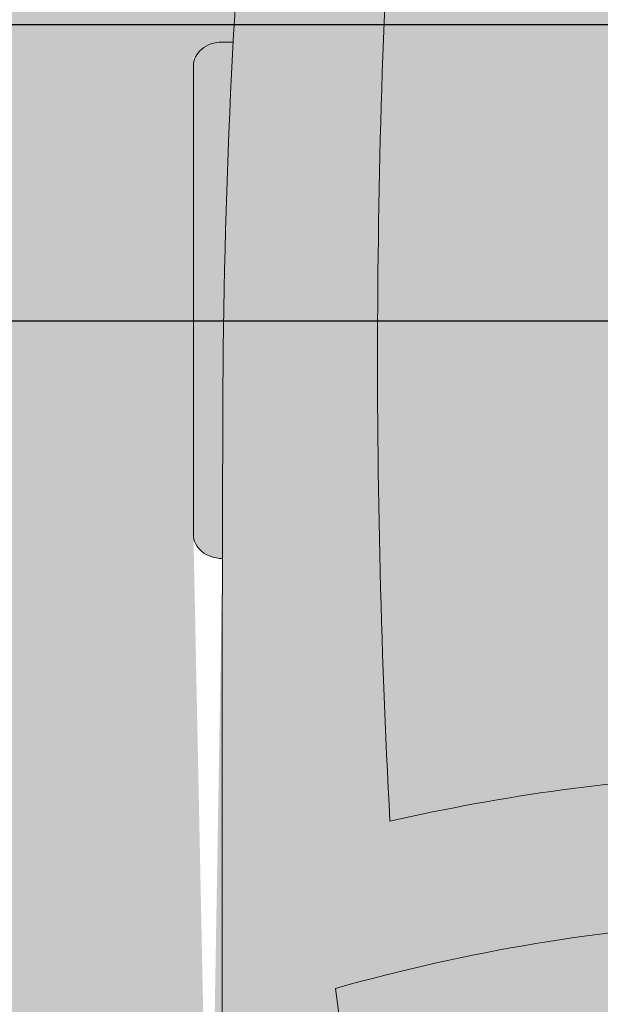
# Model space of a CAD drawing. Units: inches. Extents: x 389 to 971, y 148 to 870.
# Tile 2 of 14: x 477 to 500, y 349 to 389. Entities that reach past the tile are written whole.
import ezdxf

# ---------------------------------------------------------------- set-up
doc = ezdxf.new("R2010")
doc.units = ezdxf.units.IN
doc.header["$MEASUREMENT"] = 0
for name, color, linetype, lineweight in [('A-ANNO-DIMS', 2, 'Continuous', 18), ('C-VEHI', 8, 'Continuous', 13), ('L-GRND-BASE-PATT', 8, 'Continuous', 13)]:
    doc.layers.add(name, color=color, linetype=linetype, lineweight=lineweight)
doc.layers.add('C-VEHI-PATT', color=18, linetype='Continuous', lineweight=13, true_color=0x000000)
doc.layers.add('L-GRND-PATT', color=39, linetype='Continuous', lineweight=13, true_color=0x603913)
doc.styles.get("Standard").update_dxf_attribs({"font": 'arial.ttf'})
doc.dimstyles.get("Standard").update_dxf_attribs({"dimtxt": 8, "dimasz": 8, "dimexe": 0.18, "dimexo": 0.0625, "dimgap": 0.09, "dimtad": 0, "dimtih": 1, "dimtoh": 1, "dimdec": 0, "dimzin": 0, "dimdsep": 46, "dimlunit": 3, "dimtxsty": 'Standard', "dimcen": 0.09, "dimadec": 0, "dimazin": 0, "dimtfac": 1, "dimtdec": 0, "dimtofl": 0, "dimtmove": 0, "dimatfit": 3, "dimfxl": 1, "dimtolj": 1, "dimtzin": 0, "dimarcsym": 0})

# ---------------------------------------------------------------- blocks, each defined once
blk = doc.blocks.new('*U7')
for p, q in [((86.40615155322318, -29.35124891408145), (70.03028248535594, -31.53613089391442)), ((21.10406751471477, -37.4086304679212), (21.10406751471477, -36.83230215753756)), ((47.80016686962392, -37.39011648242107), (47.80016686962392, -37.4086304679212)), ((46.55368679439944, -38.88847654282927), (22.35054758993934, -38.88847654282927))]:
    blk.add_line(p, q)
for centre, major_axis, ratio, start_param, end_param in [((135.2911776514465, -5.387441675480715), (3.2038e-12, -81.77258453066244), 0.8423038695439492, -1.50788012981387, -1.245306111696839), ((134.4003789125684, -5.387441675478584), (4.2949e-12, -89.77745434847827), 0.8423038695439354, -1.510751403667474, -1.307889310215002), ((37.47375371777847, 593.9621830607904), (1.1693e-12, -623.3282099673584), 0.8423038695439528, -0.0593185269054384, 0.0455465850287298), ((41.19115208863322, 490.8631038926152), (1.37757e-11, -528.2339998381949), 0.8423038695440652, -0.0755983031097181, -0.0028100083537155), ((64.48199294495228, 10555.61767590795), (6.117947e-10, 10593.02630637587), 0.8423038695458146, 3.138795612625926, 3.154989602201039), ((22.35054758993934, -37.40863046792117), (2.2e-14, 1.479846074908118), 0.8423038695439758, 1.570796326794908, 3.14159265358981), ((46.55368679439944, -37.40863046792117), (2.08e-14, -1.479846074908118), 0.842303869543976, -1.69e-14, 1.570796326794884)]:
    blk.add_ellipse(centre, major_axis=major_axis, ratio=ratio, start_param=start_param, end_param=end_param)
blk = doc.blocks.new('*D53')
at = {"layer": 'A-ANNO-DIMS', "color": 0, "lineweight": -2, "transparency": 16777216}
for p, q in [((397.8910240000004, 396.9189020000002), (397.8910240000004, 404.9189020000001)), ((690.1535240000002, 388.9189020000003), (397.7110240000004, 388.9189020000002)), ((690.1535240000002, 376.9189020000001), (397.7110240000005, 376.9189020000001)), ((397.8910240000005, 368.9189020000001), (397.8910240000005, 360.918902))]:
    blk.add_line(p, q, dxfattribs=at)
at = {"layer": 'A-ANNO-DIMS', "color": 0, "transparency": 16777216}
for points in [[(396.5576906666671, 396.9189020000002), (399.2243573333337, 396.9189020000002), (397.8910240000004, 388.9189020000002)], [(396.5576906666671, 368.9189020000001), (399.2243573333338, 368.9189020000001), (397.8910240000005, 376.9189020000001)]]:
    blk.add_solid(points, dxfattribs=at)
at = {"layer": 'Defpoints', "color": 0, "transparency": 16777216}
for p in [(397.8910240000004, 388.9189020000002), (690.2160240000001, 388.9189020000003), (690.2160240000001, 376.9189020000001)]:
    blk.add_point(p, dxfattribs=at)
at = {"layer": 'A-ANNO-DIMS', "color": 0, "transparency": 16777216, "insert": (397.8910240000004, 382.9189019999999), "char_height": 8, "attachment_point": 5}
blk.add_mtext('\\A1;12', dxfattribs=at)

msp = doc.modelspace()

# ---------------------------------------------------------------- hatches: boundary and pattern name
at = {"layer": 'C-VEHI-PATT'}
h = msp.add_hatch(color=256, dxfattribs=at)
h.dxf.hatch_style = 1
edge = h.paths.add_edge_path()
edge.add_ellipse((550.9021553826709, 381.4331108862803), major_axis=(-43.99405423656321, 1.9369e-12), ratio=0.8423038695439613, start_angle=-29.43856959797762, end_angle=1.8189894035458565e-12, ccw=False)
edge.add_line((514.3535105156315, 402.059641051582), (514.3535105156315, 404.7525403567118))
edge.add_ellipse((514.3535105156316, 404.2643898676136), major_axis=(0.5795420236673633, 2e-16), ratio=0.8423038695437671, start_angle=90.00000000001334, end_angle=127.9331304598466)
edge.add_line((514.0354569934393, 404.6724605914631), (509.5535496243029, 402.1940957519602))
edge.add_ellipse((473.3138688667988, 564.9222417143382), major_axis=(196.5636751472093, 8.4793e-12), ratio=0.8423038695439335, start_angle=-80.7434339928015, end_angle=-77.44506735586577, ccw=False)
edge.add_ellipse((535.9119176052684, 201.7546502845751), major_axis=(239.1273775699096, 1.008988e-10), ratio=0.842303869543627, start_angle=100.2095389971183, end_angle=102.4446272934191)
edge.add_ellipse((979.5722266908713, 375.4013592680145), major_axis=(-488.2195497741742, 7.7268e-12), ratio=0.842303869543895, start_angle=-2.863714607837472, end_angle=2.198540565955285)
edge.add_ellipse((510.1338164488812, 299.4839331720496), major_axis=(70.3178640738586, 3.814e-12), ratio=0.8423038695439212, start_angle=94.08241069114638, end_angle=107.71995322274631, ccw=False)
edge.add_line((505.914122382133, 358.6062023341113), (522.79289864913, 358.606202334111))
edge.add_ellipse((518.5732045823792, 299.4839331720493), major_axis=(-70.31786407385354, 1.4408e-12), ratio=0.8423038695439844, start_angle=252.2800467772501, end_angle=265.91758930884987, ccw=False)
edge.add_ellipse((49.13479434038987, 375.4013592680261), major_axis=(-488.2195497741754, 2.5232e-12), ratio=0.8423038695439587, start_angle=177.8014594340444, end_angle=182.8637146078372)
edge.add_ellipse((492.795103425985, 201.7546502845724), major_axis=(239.12737756976, 4.82267e-11), ratio=0.8423038695441539, start_angle=77.5553727065425, end_angle=79.79046100284327)
edge.add_ellipse((555.3931521644682, 564.9222417143374), major_axis=(-196.5636751472384, 3.62381e-11), ratio=0.8423038695438114, start_angle=77.4450673558726, end_angle=80.74343399280832, ccw=False)
edge.add_line((519.1534714069603, 402.19409575196), (514.671564037824, 404.6724605914631))
edge.add_ellipse((514.3535105156316, 404.2643898676136), major_axis=(0.5795420236673633, 2e-16), ratio=0.8423038695437671, start_angle=52.06686954015338, end_angle=90.00000000001334)
edge.add_line((514.3535105156315, 404.7525403567118), (514.3535105156315, 402.0596410515821))
edge.add_ellipse((477.8048656485917, 381.4331108862812), major_axis=(-43.99405423656326, 6.67e-13), ratio=0.8423038695439753, start_angle=180.0000000000002, end_angle=209.4385695979796, ccw=False)
edge.add_line((521.7989198851549, 381.4331108862806), (521.7989198851549, 379.5923831537828))
edge.add_line((521.7989198851549, 379.5923831537828), (523.2258361412675, 379.5923831537828))
edge.add_ellipse((523.0896049791924, 379.1042326646847), major_axis=(0.5795420236669786, 3.601e-13), ratio=0.8423038695443263, start_angle=45.519789117397124, end_angle=89.99999999996442, ccw=False)
edge.add_line((523.4589887688404, 379.4803801228631), (527.8015488731598, 376.4548385069232))
edge.add_line((527.8015488731598, 376.4548385069232), (527.8015488731597, 364.8548231745798))
edge.add_ellipse((524.8002343791572, 364.9712406163019), major_axis=(0.279312372030448, 4.96584264291768), ratio=0.6038335755719146, start_angle=106.34259195429831, end_angle=270.9979857249735, ccw=False)
edge.add_line((521.7989198851548, 364.2715269884119), (521.7989198851549, 381.4331108862806))
edge.add_ellipse((477.8048656485917, 381.4331108862812), major_axis=(-43.99405423656326, 6.67e-13), ratio=0.8423038695439753, start_angle=180.0000000000001, end_angle=209.4385695979795)
edge.add_ellipse((550.9021553826709, 381.4331108862803), major_axis=(-43.99405423656321, 1.9369e-12), ratio=0.8423038695439613, start_angle=-29.43856959797755, end_angle=1.8539e-12)
edge.add_line((506.9081011461076, 381.43311088628), (506.9081011461074, 364.2715269884121))
edge.add_ellipse((503.9067866521049, 364.9712406163021), major_axis=(-0.2793123720310282, 4.965842642917721), ratio=0.6038335755718928, start_angle=89.00201427501901, end_angle=253.6574080456941, ccw=False)
edge.add_line((500.9054721581025, 364.8548231745812), (500.9054721581025, 376.4548385069235))
edge.add_line((500.9054721581025, 376.4548385069235), (505.3530060491612, 379.5535172937331))
edge.add_ellipse((505.61741605207, 379.1042326646849), major_axis=(-0.5795420236672051, 1.236e-13), ratio=0.842303869543997, start_angle=-89.99999999998778, end_angle=-45.51978911742469, ccw=False)
edge.add_line((505.61741605207, 379.5923831537831), (506.9081011461076, 379.5923831537831))
edge.add_line((506.9081011461076, 379.5923831537831), (506.9081011461076, 381.43311088628))
h = msp.add_hatch(color=256, dxfattribs=at)
h.dxf.hatch_style = 1
edge = h.paths.add_edge_path()
edge.add_ellipse((550.9021553826709, 381.4331108862803), major_axis=(-43.99405423656321, 1.9369e-12), ratio=0.8423038695439613, start_angle=-17.01851281727818, end_angle=1.8189894035458565e-12, ccw=False)
edge.add_line((509.5535496243029, 394.0892586662828), (509.5535496243029, 402.1940957519602))
edge.add_ellipse((473.3138688667988, 564.9222417143382), major_axis=(196.5636751472093, 8.4793e-12), ratio=0.8423038695439335, start_angle=-80.7434339928015, end_angle=-77.44506735586577, ccw=False)
edge.add_ellipse((535.9119176052684, 201.7546502845751), major_axis=(239.1273775699096, 1.008988e-10), ratio=0.842303869543627, start_angle=100.2095389971183, end_angle=102.4446272934191)
edge.add_ellipse((979.5722266908713, 375.4013592680145), major_axis=(-488.2195497741742, 7.7268e-12), ratio=0.842303869543895, start_angle=-2.863714607837472, end_angle=2.198540565955285)
edge.add_ellipse((510.1338164488812, 299.4839331720496), major_axis=(70.3178640738586, 3.814e-12), ratio=0.8423038695439212, start_angle=94.08241069114638, end_angle=107.71995322274631, ccw=False)
edge.add_line((505.914122382133, 358.6062023341113), (509.5535496243029, 358.6062023341112))
edge.add_line((509.5535496243029, 358.6062023341112), (509.5535496243029, 394.0892586662828))
edge.add_ellipse((550.9021553826709, 381.4331108862803), major_axis=(-43.99405423656321, 1.9369e-12), ratio=0.8423038695439613, start_angle=-17.01851281727824, end_angle=1.8539e-12)
edge.add_line((506.9081011461076, 381.43311088628), (506.9081011461074, 364.2715269884121))
edge.add_ellipse((503.9067866521049, 364.9712406163021), major_axis=(-0.2793123720310282, 4.965842642917721), ratio=0.6038335755718928, start_angle=89.00201427501901, end_angle=253.6574080456941, ccw=False)
edge.add_line((500.9054721581025, 364.8548231745812), (500.9054721581025, 376.4548385069235))
edge.add_line((500.9054721581025, 376.4548385069235), (505.3172273641584, 379.5285896248376))
edge.add_ellipse((505.61741605207, 379.1042326646849), major_axis=(-0.5795420236672051, 1.236e-13), ratio=0.842303869543997, start_angle=-89.99999999998778, end_angle=-45.51978911742469, ccw=False)
edge.add_line((505.61741605207, 379.5923831537831), (506.9081011461076, 379.5923831537831))
edge.add_line((506.9081011461076, 379.5923831537831), (506.9081011461076, 381.43311088628))
h = msp.add_hatch(color=256, dxfattribs=at)
h.dxf.hatch_style = 1
edge = h.paths.add_edge_path(flags=16)
edge.add_ellipse((3386.011413077446, 329.726312794031), major_axis=(-2896.629999631248, 1.069454e-10), ratio=0.8423038695494893, start_angle=-0.1208973690315247, end_angle=0.3640763488915013, ccw=False)
edge.add_line((489.3905023836935, 335.8383575186984), (486.2179253655185, 346.1978202249628))
edge.add_ellipse((8782.002602781096, 354.247254279773), major_axis=(-8295.790181758603, 9.87839e-10), ratio=0.8423038695486498, start_angle=0.0555943135052214, end_angle=0.3777641939157137)
edge.add_line((486.4665645878948, 299.5520931219791), (489.4638383140943, 311.3204429697198))
edge = h.paths.add_edge_path(flags=16)
edge.add_ellipse((512.1608573463288, 287.5825181681774), major_axis=(62.33048198263887, 2.0798e-12), ratio=0.8423038695439498, start_angle=94.8700695971331, end_angle=112.791914877584)
edge.add_line((491.3642517254777, 337.0752369161335), (489.6529508739416, 349.9015767089268))
edge.add_ellipse((510.1338164488795, 298.7862183048575), major_axis=(64.04807894948699, 3.9006e-12), ratio=0.8423038695439252, start_angle=94.27742096304979, end_angle=111.83495379670401, ccw=False)
edge.add_line((506.1068129054811, 352.6274231954524), (522.600208125781, 352.6274231954521))
edge.add_ellipse((518.5732045823798, 298.7862183048586), major_axis=(64.04807894948067, 3.24e-14), ratio=0.8423038695439885, start_angle=68.16504620328948, end_angle=85.72257903694378, ccw=False)
edge.add_line((539.05407015732, 349.9015767089259), (537.3427693057835, 337.0752369161327))
edge.add_ellipse((516.5461636849332, 287.5825181681899), major_axis=(62.33048198262021, 1.5954e-12), ratio=0.8423038695439995, start_angle=67.20808512240782, end_angle=85.12993040286212)
edge.add_line((521.0080028322477, 339.9490379899644), (507.6990181990146, 339.9490379899646))
edge = h.paths.add_edge_path(flags=16)
edge.add_ellipse((514.3535105156315, 391.3730654902235), major_axis=(-115.1512533244504, 1.8736e-12), ratio=0.8423038695439684, start_angle=76.4018653097696, end_angle=103.5981346902308)
edge.add_line((537.3427693057832, 296.3333211885938), (537.342769305783, 281.5897392316151))
edge.add_ellipse((514.3535105156313, 376.6294835332447), major_axis=(-115.1512533244486, 9.02e-13), ratio=0.8423038695439828, start_angle=76.40186530976922, end_angle=103.59813469023032, ccw=False)
edge.add_line((491.3642517254773, 281.5897392316156), (491.3642517254774, 296.3333211885945))
edge = h.paths.add_edge_path()
edge.add_ellipse((8782.002602781105, 354.2472542798386), major_axis=(-8296.949265805946, 5.39345e-11), ratio=0.8423038695428886, start_angle=0.3838667787920247, end_angle=0.5282714718170651)
edge.add_ellipse((8782.002602781105, 354.2472542798386), major_axis=(-8296.949265805946, 5.39345e-11), ratio=0.8423038695428886, start_angle=0.5282714718170651, end_angle=0.6465540970606384)
edge.add_ellipse((488.1158467995968, 260.6509346628684), major_axis=(2.318168094668909, 7.48e-14), ratio=0.8423038695439647, start_angle=180.6465540970884, end_angle=269.9999999999081)
edge.add_line((488.115846799593, 258.6983327064755), (491.3642517254771, 258.6983327064753))
edge.add_line((491.3642517254771, 258.6983327064753), (491.3642517254771, 274.201106836649))
edge.add_ellipse((493.6824198201462, 273.9438556676354), major_axis=(-2.318168094668919, 1.896e-13), ratio=0.8423038695439611, start_angle=-89.99999999999523, end_angle=4.718003765447065e-12, ccw=False)
edge.add_line((493.6824198201462, 275.8964576240284), (535.3300149439905, 275.8964576240277))
edge.add_ellipse((535.024601211114, 273.9438556676347), major_axis=(2.318168094668976, 2.946e-13), ratio=0.8423038695439647, start_angle=-7.275957614183426e-12, end_angle=89.99999999998943, ccw=False)
edge.add_line((537.342769305783, 273.9438556676347), (537.3427693057827, 258.698332706474))
edge.add_line((537.3427693057827, 258.698332706474), (540.591174231666, 258.6983327064739))
edge.add_ellipse((540.5911742316634, 260.6509346628669), major_axis=(-2.318168094668839, 2.143e-13), ratio=0.8423038695440144, start_angle=90.00000000008203, end_angle=179.3534459029346)
edge.add_ellipse((-7753.295581726658, 354.2472542799028), major_axis=(-8296.949265782761, 2.068448e-10), ratio=0.8423038695442414, start_angle=179.3534459029388, end_angle=179.3813568036815)
edge.add_ellipse((-7753.295581726658, 354.2472542799028), major_axis=(-8296.949265782761, 2.068448e-10), ratio=0.8423038695442414, start_angle=179.3813568036815, end_angle=179.4717285281828)
edge.add_ellipse((-7753.295581726658, 354.2472542799028), major_axis=(-8296.949265782761, 2.068448e-10), ratio=0.8423038695442414, start_angle=179.4717285281828, end_angle=179.6161332212082)
edge.add_ellipse((-7753.295581726658, 354.2472542799028), major_axis=(-8296.949265782761, 2.068448e-10), ratio=0.8423038695442414, start_angle=179.6161332212082, end_angle=180.090229088595)
edge.add_ellipse((-7753.295581726658, 354.2472542799028), major_axis=(-8296.949265782761, 2.068448e-10), ratio=0.8423038695442414, start_angle=180.090229088595, end_angle=180.134986576859)
edge.add_ellipse((129.8867725257751, 372.4897205359271), major_axis=(-413.7373561031673, 2.44623e-11), ratio=0.8423038695441432, start_angle=180.1806905311865, end_angle=182.1799503136479)
edge.add_ellipse((129.8867725257751, 372.4897205359271), major_axis=(-413.7373561031673, 2.44623e-11), ratio=0.8423038695441432, start_angle=182.1799503136479, end_angle=183.6504275857017)
edge.add_ellipse((492.7951034259847, 196.3854951855023), major_axis=(245.3971626940514, 1.422861e-10), ratio=0.8423038695444116, start_angle=76.21947101046817, end_angle=77.87403444768196)
edge.add_ellipse((49.13479434038987, 375.4013592680261), major_axis=(-488.2195497741754, 2.5232e-12), ratio=0.8423038695439587, start_angle=177.8014594340445, end_angle=182.8637146078372, ccw=False)
edge.add_ellipse((518.5732045823792, 299.4839331720493), major_axis=(-70.31786407385354, 1.4408e-12), ratio=0.8423038695439844, start_angle=252.2800467772501, end_angle=265.9175893088498)
edge.add_line((522.79289864913, 358.606202334111), (505.9141223821329, 358.6062023341113))
edge.add_ellipse((510.1338164488812, 299.4839331720496), major_axis=(70.3178640738586, 3.814e-12), ratio=0.8423038695439212, start_angle=94.08241069114636, end_angle=107.7199532227462)
edge.add_ellipse((979.5722266908713, 375.4013592680145), major_axis=(-488.2195497741742, 7.7268e-12), ratio=0.842303869543895, start_angle=-2.863714607837494, end_angle=2.198540565955284, ccw=False)
edge.add_ellipse((535.9119176052733, 196.3854951855018), major_axis=(-245.3971626940985, 1.013648e-10), ratio=0.8423038695442548, start_angle=-77.87403444769295, end_angle=-76.2194710104792)
edge.add_ellipse((898.8202485054873, 372.489720535918), major_axis=(413.7373561031672, 1.26113e-11), ratio=0.8423038695441164, start_angle=176.3495724142985, end_angle=177.8200496863523)
edge.add_ellipse((898.8202485054873, 372.489720535918), major_axis=(413.7373561031672, 1.26113e-11), ratio=0.8423038695441164, start_angle=177.8200496863523, end_angle=179.8643876095591)
edge.add_ellipse((8782.002602781105, 354.2472542798386), major_axis=(-8296.949265805946, 5.39345e-11), ratio=0.8423038695428886, start_angle=-0.1349865768573029, end_angle=-0.090229088593484)
edge.add_ellipse((8782.002602781105, 354.2472542798386), major_axis=(-8296.949265805946, 5.39345e-11), ratio=0.8423038695428886, start_angle=-0.090229088593484, end_angle=0.3838667787920247)
edge = h.paths.add_edge_path(flags=16)
edge.add_ellipse((-2357.304392046186, 329.7263127941099), major_axis=(2896.629999631251, 5.35614e-11), ratio=0.8423038695445265, start_angle=-0.3640763488920631, end_angle=0.1208973690309369)
edge.add_line((539.3165186475693, 335.8383575187012), (542.4890956657468, 346.1978202249727))
edge.add_ellipse((-7753.295581749842, 354.2472542800017), major_axis=(8295.790181758617, 3.2664368e-09), ratio=0.8423038695525207, start_angle=-0.37776419393310334, end_angle=-0.055594313522590255, ccw=False)
edge.add_line((542.240456443367, 299.5520931219743), (539.2431827171666, 311.3204429697195))
h = msp.add_hatch(color=256, dxfattribs=at)
h.dxf.hatch_style = 1
edge = h.paths.add_edge_path()
edge.add_ellipse((898.8202485054873, 372.489720535918), major_axis=(413.7373561031672, 1.26113e-11), ratio=0.8423038695441164, start_angle=177.8200496863524, end_angle=179.8643876095592, ccw=False)
edge.add_line((485.5047440247956, 388.2228563544795), (485.0533369751571, 388.2228563544795))
edge.add_ellipse((485.0533369751571, 387.2465553762829), major_axis=(1.159084047334488, 1.838e-13), ratio=0.8423038695439892, start_angle=89.9999999999909, end_angle=179.9999999999909)
edge.add_line((483.8942529278225, 387.2465553762829), (483.8942529278224, 368.2895347624687))
edge.add_ellipse((485.0533369751568, 368.2895347624687), major_axis=(-1.159084047334488, 1.838e-13), ratio=0.8423038695439892, start_angle=9.0871e-12, end_angle=90.00000000000905)
edge.add_line((485.0533369751553, 367.3132337842722), (485.0678379868568, 367.3132337842722))
edge.add_ellipse((8782.002602781105, 354.2472542798386), major_axis=(-8296.949265805946, 5.39345e-11), ratio=0.8423038695428886, start_angle=-0.13498657685727267, end_angle=-0.0902290885933894, ccw=False)
h = msp.add_hatch(color=256, dxfattribs=at)
h.dxf.hatch_style = 1
edge = h.paths.add_edge_path()
edge.add_ellipse((518.5732045823798, 298.7862183048586), major_axis=(64.04807894948067, 3.24e-14), ratio=0.8423038695439885, start_angle=68.16504620328955, end_angle=85.72257903694374)
edge.add_line((522.600208125781, 352.6274231954521), (506.106812905481, 352.6274231954524))
edge.add_ellipse((510.1338164488795, 298.7862183048575), major_axis=(64.04807894948699, 3.9006e-12), ratio=0.8423038695439252, start_angle=94.2774209630498, end_angle=111.834953796704)
edge.add_line((489.6529508739416, 349.9015767089268), (491.3642517254777, 337.0752369161335))
edge.add_ellipse((512.1608573463288, 287.5825181681774), major_axis=(62.33048198263887, 2.0798e-12), ratio=0.8423038695439498, start_angle=94.87006959713312, end_angle=112.79191487758399, ccw=False)
edge.add_line((507.6990181990146, 339.9490379899646), (521.0080028322477, 339.9490379899644))
edge.add_ellipse((516.5461636849332, 287.5825181681899), major_axis=(62.33048198262021, 1.5954e-12), ratio=0.8423038695439995, start_angle=67.2080851224078, end_angle=85.1299304028621, ccw=False)
edge.add_line((537.3427693057835, 337.0752369161327), (539.05407015732, 349.9015767089259))
at = {"layer": 'L-GRND-BASE-PATT'}
h = msp.add_hatch(color=256, dxfattribs=at)
h.dxf.hatch_style = 1
edge = h.paths.add_edge_path(flags=16)
edge.add_ellipse((8782.002602781105, 354.2472542798386), major_axis=(-8296.949265805946, 5.39345e-11), ratio=0.8423038695428886, start_angle=-0.0902290885933894, end_angle=0.3838667787920258, ccw=False)
edge.add_ellipse((485.0533369751568, 368.2895347624687), major_axis=(-1.159084047334488, 1.838e-13), ratio=0.8423038695439892, start_angle=9.094947017729282e-12, end_angle=90.00000000000898, ccw=False)
edge.add_line((483.8942529278224, 368.2895347624687), (483.8942529278225, 387.6039063360424))
edge.add_ellipse((485.0533369751571, 387.2465553762829), major_axis=(1.159084047334488, 1.838e-13), ratio=0.8423038695439892, start_angle=89.99999999999102, end_angle=179.9999999999909, ccw=False)
edge.add_line((485.0533369751572, 388.2228563544795), (485.5047440247956, 388.2228563544795))
edge.add_ellipse((898.8202485054873, 372.489720535918), major_axis=(413.7373561031672, 1.26113e-11), ratio=0.8423038695441164, start_angle=176.3495724142986, end_angle=177.8200496863524, ccw=False)
edge.add_ellipse((535.9119176052733, 196.3854951855018), major_axis=(-245.3971626940985, 1.013648e-10), ratio=0.8423038695442548, start_angle=-77.87403444769302, end_angle=-76.2194710104792, ccw=False)
edge.add_ellipse((535.9119176052684, 201.7546502845751), major_axis=(239.1273775699096, 1.008988e-10), ratio=0.842303869543627, start_angle=100.20953899711827, end_angle=102.44462729341922, ccw=False)
edge.add_ellipse((473.3138688667988, 564.9222417143382), major_axis=(196.5636751472093, 8.4793e-12), ratio=0.8423038695439335, start_angle=-80.74343399280163, end_angle=-77.44506735586587)
edge.add_line((509.5535496243029, 402.1940957519602), (514.3535105156315, 404.8483349684994))
edge.add_line((514.3535105156315, 404.8483349684994), (514.3535105156315, 404.7971763262221))
edge.add_ellipse((514.3535105156316, 404.2643898676136), major_axis=(0.5795420236673633, 2e-16), ratio=0.8423038695437671, start_angle=52.06686954015339, end_angle=90.00000000001342, ccw=False)
edge.add_line((514.671564037824, 404.672460591463), (519.1534714069603, 402.19409575196))
edge.add_ellipse((555.3931521644682, 564.9222417143374), major_axis=(-196.5636751472384, 3.62381e-11), ratio=0.8423038695438114, start_angle=77.44506735587258, end_angle=80.74343399280833)
edge.add_ellipse((492.795103425985, 201.7546502845724), major_axis=(239.12737756976, 4.82267e-11), ratio=0.8423038695441539, start_angle=77.55537270654253, end_angle=79.7904610028433, ccw=False)
edge.add_ellipse((492.7951034259847, 196.3854951855023), major_axis=(245.3971626940514, 1.422861e-10), ratio=0.8423038695444116, start_angle=76.21947101046823, end_angle=77.87403444768199, ccw=False)
edge.add_ellipse((129.8867725257751, 372.4897205359271), major_axis=(-413.7373561031673, 2.44623e-11), ratio=0.8423038695441432, start_angle=182.179950313648, end_angle=183.6504275857018, ccw=False)
edge.add_line((543.2022770064673, 388.2228563544788), (544.0779382625514, 388.2228563544787))
edge.add_ellipse((543.6536840561057, 387.2465553762822), major_axis=(-1.159084047334545, 1.527e-13), ratio=0.8423038695438989, start_angle=180.0000000000075, end_angle=270.00000000000756, ccw=False)
edge.add_line((544.8127681034401, 387.2465553762826), (544.8127681034399, 367.9321838027083))
edge.add_ellipse((543.6536840561054, 368.2895347624679), major_axis=(1.159084047334544, 7.24e-14), ratio=0.8423038695439478, start_angle=269.9999999999964, end_angle=359.9999999999964, ccw=False)
edge.add_ellipse((-7753.295581726658, 354.2472542799028), major_axis=(-8296.949265782761, 2.068448e-10), ratio=0.8423038695442414, start_angle=179.6161332212083, end_angle=180.0902290885951, ccw=False)
edge.add_line((543.3912265319653, 298.6607849184036), (544.0779382625504, 298.6607849184036))
edge.add_ellipse((543.6536840561046, 297.6844839402071), major_axis=(1.159084047334431, 1.769e-13), ratio=0.8423038695439814, start_angle=-1.1482370609883219e-11, end_angle=89.99999999999119, ccw=False)
edge.add_line((544.8127681034391, 297.684483940207), (544.8127681034387, 278.3701123666333))
edge.add_ellipse((543.6536840561043, 278.727463326393), major_axis=(-1.159084047334431, 2.574e-13), ratio=0.8423038695440306, start_angle=90.00000000001268, end_angle=180.0000000000099, ccw=False)
edge.add_line((543.6536840561045, 277.7511623481965), (543.1566278692261, 277.7511623481965))
edge.add_ellipse((-7753.295581726658, 354.2472542799028), major_axis=(-8296.949265782761, 2.068448e-10), ratio=0.8423038695442414, start_angle=179.3813568036816, end_angle=179.4717285281829, ccw=False)
edge.add_ellipse((542.4236240941387, 263.2762864208561), major_axis=(-1.738626071001761, 2.132e-13), ratio=0.8423038695439151, start_angle=179.3717627838137, end_angle=248.464756601011, ccw=False)
edge.add_ellipse((-7753.875123750511, 354.2472542780016), major_axis=(-8298.740341433751, 2.4782644722e-06), ratio=0.8423038662721074, start_angle=179.3534459200609, end_angle=179.3717628008941, ccw=False)
edge.add_ellipse((540.0116322079951, 260.6509346628677), major_axis=(-4.109243751168186, 2.384e-13), ratio=0.842303869543976, start_angle=90.0000000000635, end_angle=179.3534459029233, ccw=False)
edge.add_line((540.0116322079991, 257.1897027503593), (488.6953888232593, 257.1897027503609))
edge.add_ellipse((488.6953888232669, 260.6509346628715), major_axis=(4.10924375117072, 1.262e-13), ratio=0.8423038695439824, start_angle=180.6465540970565, end_angle=269.9999999998589, ccw=False)
edge.add_ellipse((8782.582144816053, 354.2472542821698), major_axis=(-8298.740341477976, 1.8591886369e-06), ratio=0.8423038720186145, start_angle=0.6282372290784792, end_angle=0.6465541099116194, ccw=False)
edge.add_ellipse((486.2833969371199, 263.2762864208594), major_axis=(-1.738626071002378, 2.7e-13), ratio=0.8423038695439394, start_angle=-68.46475649596817, end_angle=0.6282372161796275, ccw=False)
edge.add_ellipse((8782.002602781105, 354.2472542798386), major_axis=(-8296.949265805946, 5.39345e-11), ratio=0.8423038695428886, start_angle=0.5282714718171064, end_angle=0.6465540970606867, ccw=False)
edge.add_line((485.5503931620382, 277.7511623481972), (484.6290827687102, 277.7511623481972))
edge.add_ellipse((485.0533369751559, 278.7274633263938), major_axis=(-1.159084047334545, 3.11e-13), ratio=0.8423038695439968, start_angle=1.5404566511278972e-11, end_angle=90.000000000012, ccw=False)
edge.add_line((483.8942529278214, 278.7274633263938), (483.8942529278216, 298.0418348999672))
edge.add_ellipse((485.053336975156, 297.6844839402078), major_axis=(1.159084047334488, 1.025e-13), ratio=0.8423038695440382, start_angle=89.99999999999488, end_angle=179.9999999999949, ccw=False)
edge = h.paths.add_edge_path(flags=0)
edge.add_ellipse((8782.002602781096, 354.247254279773), major_axis=(-8295.790181758603, 9.87839e-10), ratio=0.8423038695486498, start_angle=0.05559431350519617, end_angle=0.37776419391582294, ccw=False)
edge.add_line((486.2179253655185, 346.1978202249628), (489.3905023836935, 335.8383575186984))
edge.add_ellipse((3386.011413077446, 329.726312794031), major_axis=(-2896.629999631248, 1.069454e-10), ratio=0.8423038695494893, start_angle=-0.1208973690315206, end_angle=0.3640763488915184)
edge.add_line((489.4638383140943, 311.3204429697198), (486.4665645878948, 299.5520931219791))
edge = h.paths.add_edge_path(flags=0)
edge.add_ellipse((514.3535105156315, 391.3730654902235), major_axis=(-115.1512533244504, 1.8736e-12), ratio=0.8423038695439684, start_angle=76.4018653097696, end_angle=103.5981346902308)
edge.add_line((537.3427693057832, 296.3333211885938), (537.342769305783, 281.5897392316151))
edge.add_ellipse((514.3535105156313, 376.6294835332447), major_axis=(-115.1512533244486, 9.02e-13), ratio=0.8423038695439828, start_angle=76.40186530976922, end_angle=103.59813469023032, ccw=False)
edge.add_line((491.3642517254773, 281.5897392316156), (491.3642517254774, 296.3333211885945))
edge = h.paths.add_edge_path(flags=0)
edge.add_line((491.3642517254777, 337.0752369161334), (489.6529508739416, 349.9015767089268))
edge.add_ellipse((510.1338164488795, 298.7862183048575), major_axis=(64.04807894948699, 3.9006e-12), ratio=0.8423038695439252, start_angle=94.27742096304979, end_angle=111.83495379670401, ccw=False)
edge.add_line((506.106812905481, 352.6274231954524), (522.600208125781, 352.6274231954521))
edge.add_ellipse((518.5732045823798, 298.7862183048586), major_axis=(64.04807894948067, 3.24e-14), ratio=0.8423038695439885, start_angle=68.16504620328948, end_angle=85.72257903694378, ccw=False)
edge.add_line((539.05407015732, 349.9015767089259), (537.3427693057835, 337.0752369161327))
edge.add_ellipse((516.5461636849332, 287.5825181681899), major_axis=(62.33048198262021, 1.5954e-12), ratio=0.8423038695439995, start_angle=67.20808512240782, end_angle=85.12993040286212)
edge.add_line((521.0080028322477, 339.9490379899644), (507.6990181990146, 339.9490379899646))
edge.add_ellipse((512.1608573463288, 287.5825181681774), major_axis=(62.33048198263887, 2.0798e-12), ratio=0.8423038695439498, start_angle=94.8700695971331, end_angle=112.791914877584)
edge = h.paths.add_edge_path(flags=0)
edge.add_ellipse((493.6824198201462, 273.9438556676354), major_axis=(-2.318168094668919, 1.896e-13), ratio=0.8423038695439611, start_angle=-89.99999999999523, end_angle=4.718003765447065e-12, ccw=False)
edge.add_line((493.6824198201462, 275.8964576240284), (535.3743409680425, 275.8964576240277))
edge.add_ellipse((535.024601211114, 273.9438556676347), major_axis=(2.318168094668976, 2.946e-13), ratio=0.8423038695439647, start_angle=-7.275957614183426e-12, end_angle=89.99999999998943, ccw=False)
edge.add_line((537.342769305783, 273.9438556676347), (537.3427693057827, 258.698332706474))
edge.add_line((537.3427693057827, 258.698332706474), (540.5911742316662, 258.6983327064739))
edge.add_ellipse((540.5911742316634, 260.6509346628669), major_axis=(-2.318168094668839, 2.143e-13), ratio=0.8423038695440144, start_angle=90.00000000008203, end_angle=179.3534459029346)
edge.add_line((540.5911742316662, 258.6983327064739), (487.7691399811528, 258.6983327064755))
edge.add_ellipse((488.1158467995968, 260.6509346628684), major_axis=(2.318168094668909, 7.48e-14), ratio=0.8423038695439647, start_angle=180.6465540970884, end_angle=269.9999999999081)
edge.add_line((488.1158467995931, 258.6983327064755), (491.3642517254771, 258.6983327064754))
edge.add_line((491.3642517254771, 258.6983327064754), (491.3642517254771, 274.2384428182294))
h.paths.add_polyline_path([(746.1375687288224, 327.3223047166553), (750.1400147212453, 327.3223047166553), (750.1400147212453, 326.2830696147227), (798.1693712998389, 326.2830696147227), (798.1693712998389, 327.3223047166553), (802.1718172922616, 327.3223047166553), (802.1718172922616, 309.9783792024682, -0.1904762075443491), (746.1375687288224, 309.9783668090107)], flags=16)
h.paths.add_polyline_path([(782.1595875801748, 313.5684994305933), (782.1595893317732, 309.0414930416419, -0.0496282101666581), (766.1497986905329, 309.0414910503953), (766.1498004421323, 313.5684994305933)], flags=0)
h.paths.add_polyline_path([(755.1858908233534, 344.9352232902417), (755.1858908233534, 373.916311072083), (788.1243995226009, 373.916311072083), (788.1243995226009, 344.9352232902417)], flags=16)
h.paths.add_polyline_path([(757.1858908233535, 346.9352232902417), (757.1858908233535, 371.916311072083), (786.1243995226009, 371.916311072083), (786.1243995226009, 346.9352232902417)], flags=0)
h.paths.add_polyline_path([(803.6445810111745, 338.4878931208803), (803.6445810111745, 342.4903391133031), (804.6838161131072, 342.4903391133031), (804.6838161131072, 390.5196956918968), (803.6445810111748, 390.5196956918968), (803.6445810111748, 394.5221416843196), (820.9885065253617, 394.5221416843196, -0.1904762075443491), (820.9885189188192, 338.4878931208803)], flags=16)
h.paths.add_polyline_path([(806.8706930931005, 326.6963103558256), (806.4254411777042, 327.1415622712219), (806.4723791864895, 326.6297175483474)], flags=16)
h.paths.add_polyline_path([(822.0328146004263, 317.4007976138144), (822.1941503181826, 317.8932883068639), (821.562628166435, 317.9885306563034)], flags=16)
h.paths.add_polyline_path([(817.3983862972365, 358.5001248341902), (817.3983862972365, 374.5099119722327), (821.9253926861879, 374.5099137238312, -0.049628210166658), (821.9253946774346, 358.5001230825909)], flags=0)
h.paths.add_polyline_path([(808.1446344648577, 418.9736619306146), (808.2246858861593, 418.5632188717996), (808.5395491501399, 418.5787472453325)], flags=16)
h.paths.add_polyline_path([(820.3158762739024, 412.6690288868844), (820.4772119916585, 413.161519579934), (819.8456898399113, 413.2567619293735)], flags=16)
h.paths.add_polyline_path([(466.3155093563569, 235.5246322146605), (517.3806533266912, 235.5246322146605), (517.3806533266912, 244.4269231682286), (466.3155093563569, 244.4269231682286)], flags=24)
h.paths.add_polyline_path([(739.8737195480014, 256.2000079819968), (815.4040239338423, 256.2000079819968), (815.4040239338423, 265.3453807094367), (739.8737195480014, 265.3453807094367)], flags=24)
h.paths.add_polyline_path([(750.6081538187397, 393.6666679930368), (791.5680640722773, 393.6666679930368), (791.5680640722773, 412.3933175868746), (750.6081538187397, 412.3933175868746)], flags=24)
h.paths.add_polyline_path([(438.9630812812552, 410.0618566955462), (484.6203810968238, 410.0618566955462), (484.6203810968238, 429.1217352891893), (438.9630812812552, 429.1217352891893)], flags=24)
edge = h.paths.add_edge_path()
edge.add_line((839.2160244416713, 285.6445131961097), (611.8786784019748, 285.6445131961099))
edge.add_line((611.8786784019748, 285.6445131961099), (604.3870116090119, 285.6445131961097))
edge.add_line((604.3870116090119, 285.6445131961097), (595.3870116090119, 285.6445131961097))
edge.add_line((595.3870116090119, 285.6445131961097), (595.3870116090118, 370.1553848722774))
edge.add_line((595.3870116090118, 370.1553848722774), (604.0816928471932, 370.1553848722774))
edge.add_line((604.0816928471932, 370.1553848722774), (604.0816928471932, 371.3788335667469))
edge.add_line((604.0816928471932, 371.3788335667469), (632.0194586761203, 371.3788335667469))
edge.add_arc((604.0816928471932, 370.1553848722773), 27.96454158787471, 2.507490703587644, 90.00000000000003)
edge.add_line((604.0816928471932, 398.1199264601519), (599.8870116090108, 398.1652144688576))
edge.add_line((599.8870116090108, 398.1652144688576), (604.4225424425357, 398.1652144688576))
edge.add_arc((604.4225424425357, 428.4020866923496), 30.23687222349201, 270.0000000000002, 357.492509296413)
edge.add_line((634.6304631740308, 427.0792235325719), (604.4225424425357, 427.0792235325719))
edge.add_line((604.4225424425357, 427.0792235325719), (604.4225424425357, 428.4020866923497))
edge.add_line((604.4225424425357, 428.4020866923497), (599.8870116090119, 428.4020866923497))
edge.add_line((599.8870116090119, 428.4020866923497), (595.3870116090116, 428.4020866923497))
edge.add_line((595.3870116090116, 428.4020866923497), (595.3870116090118, 434.6445131961097))
edge.add_line((595.3870116090118, 434.6445131961097), (585.0790669792458, 434.6445131961097))
edge.add_line((585.0790669792458, 434.6445131961097), (540.3921730610418, 434.6445131961097))
edge.add_line((540.3921730610418, 434.6445131961097), (526.712508448134, 434.6445131961097))
edge.add_line((526.712508448134, 434.6445131961097), (488.4094553949635, 434.6445131961097))
edge.add_line((488.4094553949635, 434.6445131961097), (432.2160244416713, 434.6445131961097))
edge.add_line((432.2160244416713, 434.6445131961097), (432.2160244416713, 243.6445131961098))
edge.add_line((432.2160244416713, 243.6445131961098), (437.2160244416714, 243.6445131961098))
edge.add_line((437.2160244416714, 243.6445131961098), (437.2160244416714, 234.6445131961098))
edge.add_line((437.2160244416714, 234.6445131961098), (581.2160244416713, 234.6445131961098))
edge.add_line((581.2160244416713, 234.6445131961098), (581.2160244416713, 238.6445131961097))
edge.add_line((581.2160244416713, 238.6445131961097), (581.2160244416713, 243.6445131961098))
edge.add_line((581.2160244416713, 243.6445131961098), (590.2160244416713, 243.6445131961098))
edge.add_line((590.2160244416713, 243.6445131961098), (590.2160244416713, 238.6445131961097))
edge.add_line((590.2160244416713, 238.6445131961097), (839.2160244416713, 238.6445131961098))
edge.add_line((839.2160244416713, 238.6445131961098), (839.2160244416713, 285.6445131961097))
at = {"layer": 'L-GRND-PATT'}
h = msp.add_hatch(dxfattribs=at)
h.set_pattern_fill('EARTH', color=256, angle=45)
h.set_pattern_definition([(45, (0, 0), (0, 8.980256121069154), [6.349999999999999, -6.349999999999999]), (45, (-1.683798022700466, 1.683798022700466), (0, 8.980256121069154), [6.349999999999999, -6.349999999999999]), (45, (-3.367596045400933, 3.367596045400933), (0, 8.980256121069154), [6.349999999999999, -6.349999999999999]), (135, (-3.367596045400933, 4.490128060534576), (-8.980256121069154, 0), [6.349999999999999, -6.349999999999999]), (135, (-1.683798022700466, 6.173926083235043), (-8.980256121069154, 0), [6.349999999999999, -6.349999999999999]), (135, (0, 7.85772410593551), (-8.980256121069154, 0), [6.349999999999999, -6.349999999999999])])
h.paths.add_polyline_path([(432.2160244416713, 243.6445131961098), (437.2160244416714, 243.6445131961098), (437.2160244416714, 234.6445131961098), (581.2160244416713, 234.6445131961098), (581.2160244416713, 238.6445131961097), (581.2160244416713, 243.6445131961098), (590.2160244416713, 243.6445131961098), (590.2160244416713, 238.6445131961097), (839.2160244416713, 238.6445131961098), (839.2160244416712, 285.6445131961097), (810.0513609197296, 285.6445131961097), (733.8056934525983, 285.6445131961099), (684.2433676403508, 285.6445131961098), (611.8786784019748, 285.6445131961099), (604.3870116090119, 285.6445131961097), (595.3870116090119, 285.6445131961097), (595.3870116090118, 370.1553848722774), (604.0816928471932, 370.1553848722774), (604.0816928471932, 371.3788335667469), (632.0194586761203, 371.3788335667469, 0.4014527144963568), (604.0816928471932, 398.119926460152), (599.8870116090127, 398.1652144688576), (604.4225424425357, 398.1652144688576, 0.4014527144963579), (634.6304631740308, 427.0792235325719), (604.4225424425357, 427.0792235325719), (604.4225424425357, 428.4020866923497), (599.8870116090119, 428.4020866923497), (595.3870116090116, 428.4020866923497), (595.3870116090118, 434.6445131961097), (585.0790669792458, 434.6445131961097), (540.3921730610418, 434.6445131961097), (526.712508448134, 434.6445131961097), (488.4094553949635, 434.6445131961097), (432.2160244416713, 434.6445131961097)])
edge = h.paths.add_edge_path(flags=16)
edge.add_line((483.8942529278214, 278.7274633263938), (483.8942529278216, 298.2563878122772))
edge.add_ellipse((485.053336975156, 297.6844839402078), major_axis=(1.159084047334488, 1.025e-13), ratio=0.8423038695440382, start_angle=89.99999999999488, end_angle=179.9999999999949, ccw=False)
edge.add_ellipse((8782.002602781105, 354.2472542798386), major_axis=(-8296.949265805946, 5.39345e-11), ratio=0.8423038695428886, start_angle=-0.0902290885933894, end_angle=0.3838667787920258, ccw=False)
edge.add_ellipse((485.0533369751568, 368.2895347624687), major_axis=(-1.159084047334488, 1.838e-13), ratio=0.8423038695439892, start_angle=9.094947017729282e-12, end_angle=90.00000000000898, ccw=False)
edge.add_line((483.8942529278224, 368.2895347624687), (483.8942529278225, 387.8184592483523))
edge.add_ellipse((485.0533369751571, 387.2465553762829), major_axis=(1.159084047334488, 1.838e-13), ratio=0.8423038695439892, start_angle=89.99999999999102, end_angle=179.9999999999909, ccw=False)
edge.add_ellipse((898.8202485054873, 372.489720535918), major_axis=(413.7373561031672, 1.26113e-11), ratio=0.8423038695441164, start_angle=176.3495724142986, end_angle=177.8200496863524, ccw=False)
edge.add_ellipse((535.9119176052733, 196.3854951855018), major_axis=(-245.3971626940985, 1.013648e-10), ratio=0.8423038695442548, start_angle=-77.87403444769302, end_angle=-76.2194710104792, ccw=False)
edge.add_ellipse((535.9119176052684, 201.7546502845751), major_axis=(239.1273775699096, 1.008988e-10), ratio=0.842303869543627, start_angle=100.20953899711827, end_angle=102.44462729341922, ccw=False)
edge.add_ellipse((473.3138688667988, 564.9222417143382), major_axis=(196.5636751472093, 8.4793e-12), ratio=0.8423038695439335, start_angle=-80.74343399280163, end_angle=-77.44506735586587)
edge.add_line((509.5535496243029, 402.1940957519602), (514.3535105156316, 404.8483349684994))
edge.add_line((514.3535105156316, 404.8483349684994), (519.1534714069603, 402.19409575196))
edge.add_ellipse((555.3931521644682, 564.9222417143374), major_axis=(-196.5636751472384, 3.62381e-11), ratio=0.8423038695438114, start_angle=77.44506735587258, end_angle=80.74343399280833)
edge.add_ellipse((492.795103425985, 201.7546502845724), major_axis=(239.12737756976, 4.82267e-11), ratio=0.8423038695441539, start_angle=77.55537270654253, end_angle=79.7904610028433, ccw=False)
edge.add_ellipse((492.7951034259847, 196.3854951855023), major_axis=(245.3971626940514, 1.422861e-10), ratio=0.8423038695444116, start_angle=76.21947101046823, end_angle=77.87403444768199, ccw=False)
edge.add_ellipse((129.8867725257751, 372.4897205359271), major_axis=(-413.7373561031673, 2.44623e-11), ratio=0.8423038695441432, start_angle=182.179950313648, end_angle=183.6504275857018, ccw=False)
edge.add_line((543.2022770064673, 388.2228563544789), (544.3326597711041, 388.2228563544786))
edge.add_ellipse((543.6536840561057, 387.2465553762822), major_axis=(-1.159084047334545, 1.527e-13), ratio=0.8423038695438989, start_angle=180.0000000000075, end_angle=270.00000000000756, ccw=False)
edge.add_line((544.8127681034401, 387.2465553762825), (544.8127681034399, 367.7176308903986))
edge.add_ellipse((543.6536840561054, 368.2895347624679), major_axis=(1.159084047334544, 7.24e-14), ratio=0.8423038695439478, start_angle=269.9999999999964, end_angle=359.9999999999964, ccw=False)
edge.add_ellipse((-7753.295581726658, 354.2472542799028), major_axis=(-8296.949265782761, 2.068448e-10), ratio=0.8423038695442414, start_angle=179.6161332212083, end_angle=180.0902290885951, ccw=False)
edge.add_ellipse((543.6536840561046, 297.6844839402071), major_axis=(1.159084047334431, 1.769e-13), ratio=0.8423038695439814, start_angle=-1.1482370609883219e-11, end_angle=89.99999999999119, ccw=False)
edge.add_line((544.8127681034391, 297.6844839402071), (544.8127681034387, 278.1555594543235))
edge.add_ellipse((543.6536840561043, 278.727463326393), major_axis=(-1.159084047334431, 2.574e-13), ratio=0.8423038695440306, start_angle=90.00000000001268, end_angle=180.0000000000099, ccw=False)
edge.add_ellipse((-7753.295581726658, 354.2472542799028), major_axis=(-8296.949265782761, 2.068448e-10), ratio=0.8423038695442414, start_angle=179.3813568036816, end_angle=179.4717285281829, ccw=False)
edge.add_ellipse((542.4236240941387, 263.2762864208561), major_axis=(-1.738626071001761, 2.132e-13), ratio=0.8423038695439151, start_angle=179.3717627838137, end_angle=248.464756601011, ccw=False)
edge.add_ellipse((-7753.875123750511, 354.2472542780016), major_axis=(-8298.740341433751, 2.4782644722e-06), ratio=0.8423038662721074, start_angle=179.3534459200609, end_angle=179.3717628008941, ccw=False)
edge.add_ellipse((540.0116322079951, 260.6509346628677), major_axis=(-4.109243751168186, 2.384e-13), ratio=0.842303869543976, start_angle=90.0000000000635, end_angle=179.3534459029233, ccw=False)
edge.add_line((540.0116322079989, 257.1897027503593), (488.0808074948215, 257.1897027503609))
edge.add_ellipse((488.6953888232669, 260.6509346628715), major_axis=(4.10924375117072, 1.262e-13), ratio=0.8423038695439824, start_angle=180.6465540970565, end_angle=269.9999999998589, ccw=False)
edge.add_ellipse((8782.582144816053, 354.2472542821698), major_axis=(-8298.740341477976, 1.8591886369e-06), ratio=0.8423038720186145, start_angle=0.6282372290784792, end_angle=0.6465541099116194, ccw=False)
edge.add_ellipse((486.2833969371199, 263.2762864208594), major_axis=(-1.738626071002378, 2.7e-13), ratio=0.8423038695439394, start_angle=-68.46475649596817, end_angle=0.6282372161796275, ccw=False)
edge.add_ellipse((8782.002602781105, 354.2472542798386), major_axis=(-8296.949265805946, 5.39345e-11), ratio=0.8423038695428886, start_angle=0.5282714718171064, end_angle=0.6465540970606867, ccw=False)
edge.add_line((485.5503931620382, 277.7511623481972), (484.3743612601578, 277.7511623481972))
edge.add_ellipse((485.0533369751559, 278.7274633263938), major_axis=(-1.159084047334545, 3.11e-13), ratio=0.8423038695439968, start_angle=1.5404566511278972e-11, end_angle=90.000000000012, ccw=False)
edge = h.paths.add_edge_path(flags=0)
edge.add_ellipse((488.1158467995968, 260.6509346628684), major_axis=(2.318168094668909, 7.48e-14), ratio=0.8423038695439647, start_angle=180.6465540970884, end_angle=269.9999999999081)
edge.add_line((488.1158467995933, 258.6983327064755), (491.3642517254771, 258.6983327064753))
edge.add_line((491.3642517254771, 258.6983327064753), (491.3642517254771, 274.4686391213292))
edge.add_ellipse((493.6824198201462, 273.9438556676354), major_axis=(-2.318168094668919, 1.896e-13), ratio=0.8423038695439611, start_angle=-89.99999999999523, end_angle=4.718003765447065e-12, ccw=False)
edge.add_line((493.6824198201462, 275.8964576240284), (535.6476346230087, 275.8964576240277))
edge.add_ellipse((535.024601211114, 273.9438556676347), major_axis=(2.318168094668976, 2.946e-13), ratio=0.8423038695439647, start_angle=-7.275957614183426e-12, end_angle=89.99999999998943, ccw=False)
edge.add_line((537.342769305783, 273.9438556676347), (537.3427693057827, 258.698332706474))
edge.add_line((537.3427693057827, 258.698332706474), (541.2086129152347, 258.6983327064739))
edge.add_ellipse((540.5911742316634, 260.6509346628669), major_axis=(-2.318168094668839, 2.143e-13), ratio=0.8423038695440144, start_angle=90.00000000008203, end_angle=179.3534459029347, ccw=False)
edge.add_line((540.5911742316662, 258.6983327064739), (487.4984081160257, 258.6983327064755))
edge = h.paths.add_edge_path(flags=0)
edge.add_line((491.3642517254773, 281.5897392316156), (491.3642517254774, 296.3333211885945))
edge.add_ellipse((514.3535105156315, 391.3730654902235), major_axis=(-115.1512533244504, 1.8736e-12), ratio=0.8423038695439684, start_angle=76.4018653097696, end_angle=103.5981346902308)
edge.add_line((537.3427693057832, 296.3333211885938), (537.342769305783, 281.5897392316151))
edge.add_ellipse((514.3535105156313, 376.6294835332447), major_axis=(-115.1512533244486, 9.02e-13), ratio=0.8423038695439828, start_angle=76.40186530976922, end_angle=103.59813469023032, ccw=False)
edge = h.paths.add_edge_path(flags=0)
edge.add_ellipse((8782.002602781096, 354.247254279773), major_axis=(-8295.790181758603, 9.87839e-10), ratio=0.8423038695486498, start_angle=0.05559431350519617, end_angle=0.37776419391582294, ccw=False)
edge.add_line((486.2179253655185, 346.1978202249628), (489.3905023836935, 335.8383575186985))
edge.add_ellipse((3386.011413077446, 329.726312794031), major_axis=(-2896.629999631248, 1.069454e-10), ratio=0.8423038695494893, start_angle=-0.1208973690315206, end_angle=0.3640763488915184)
edge.add_line((489.4638383140943, 311.3204429697198), (486.4665645878948, 299.5520931219782))
edge = h.paths.add_edge_path(flags=0)
edge.add_line((491.3642517254777, 337.0752369161334), (489.6529508739416, 349.9015767089268))
edge.add_ellipse((510.1338164488795, 298.7862183048575), major_axis=(64.04807894948699, 3.9006e-12), ratio=0.8423038695439252, start_angle=94.27742096304979, end_angle=111.83495379670401, ccw=False)
edge.add_line((506.106812905481, 352.6274231954524), (522.600208125781, 352.6274231954521))
edge.add_ellipse((518.5732045823798, 298.7862183048586), major_axis=(64.04807894948067, 3.24e-14), ratio=0.8423038695439885, start_angle=68.16504620328948, end_angle=85.72257903694378, ccw=False)
edge.add_line((539.05407015732, 349.9015767089259), (537.3427693057835, 337.0752369161327))
edge.add_ellipse((516.5461636849332, 287.5825181681899), major_axis=(62.33048198262021, 1.5954e-12), ratio=0.8423038695439995, start_angle=67.20808512240782, end_angle=85.12993040286212)
edge.add_line((521.0080028322477, 339.9490379899644), (507.6990181990145, 339.9490379899646))
edge.add_ellipse((512.1608573463288, 287.5825181681774), major_axis=(62.33048198263887, 2.0798e-12), ratio=0.8423038695439498, start_angle=94.8700695971331, end_angle=112.791914877584)
h.paths.add_polyline_path([(466.3155093563569, 235.5246322146605), (517.3806533266912, 235.5246322146605), (517.3806533266912, 244.4269231682286), (466.3155093563569, 244.4269231682286)], flags=24)
h.paths.add_polyline_path([(739.8737195480014, 256.2000079819968), (815.4040239338423, 256.2000079819968), (815.4040239338423, 265.3453807094367), (739.8737195480014, 265.3453807094367)], flags=24)
h.paths.add_polyline_path([(438.9630812812552, 410.0618566955462), (484.6203810968238, 410.0618566955462), (484.6203810968238, 429.1217352891893), (438.9630812812552, 429.1217352891893)], flags=24)

# ---------------------------------------------------------------- block references
at = {"layer": 'C-VEHI', "xscale": 0.7832463571634928, "yscale": 0.7832463571634928, "zscale": 0.7832463571634928, "rotation": 269.9999999999993}
msp.add_blockref('*U7', (514.3535105156318, 404.7525403567118), dxfattribs=at)

# ---------------------------------------------------------------- dimensions: what is measured, and where the dimension line sits
at = {"layer": 'A-ANNO-DIMS'}
dim = msp.add_linear_dim(base=(397.8910240000004, 388.9189020000002), p1=(690.216024, 376.918902), p2=(690.216024, 388.918902), angle=90, dimstyle='Standard', override={"dimdec": 0, "dimlfac": 1, "dimrnd": 0, "dimzin": 0, "dimdsep": 46, "dimlunit": 2}, dxfattribs=at)
dim.commit()
dim.dimension.update_dxf_attribs({"geometry": '*D53', "text_midpoint": (397.8910240000004, 382.9189019999999)})

doc.saveas('drawing.dxf')
